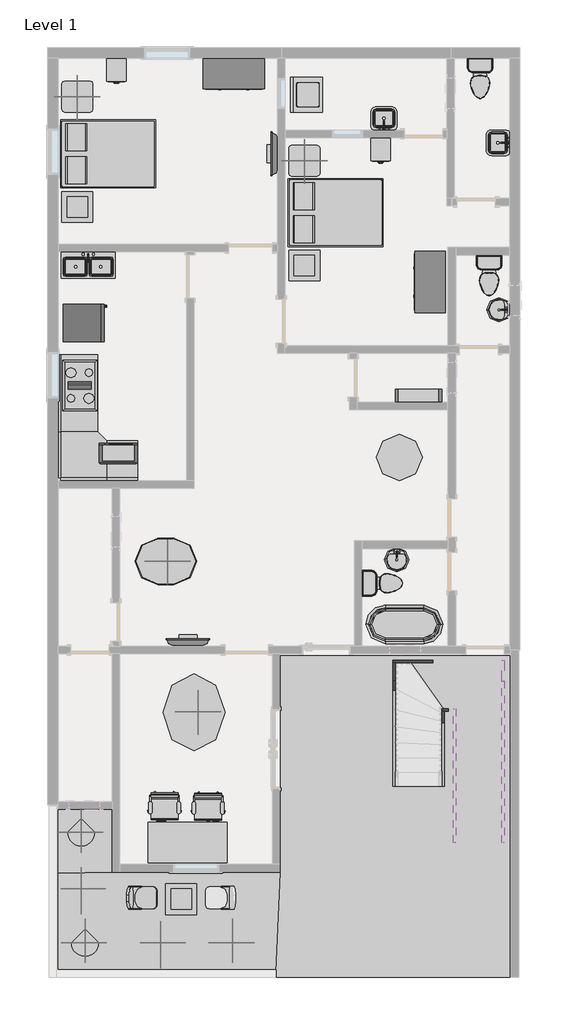
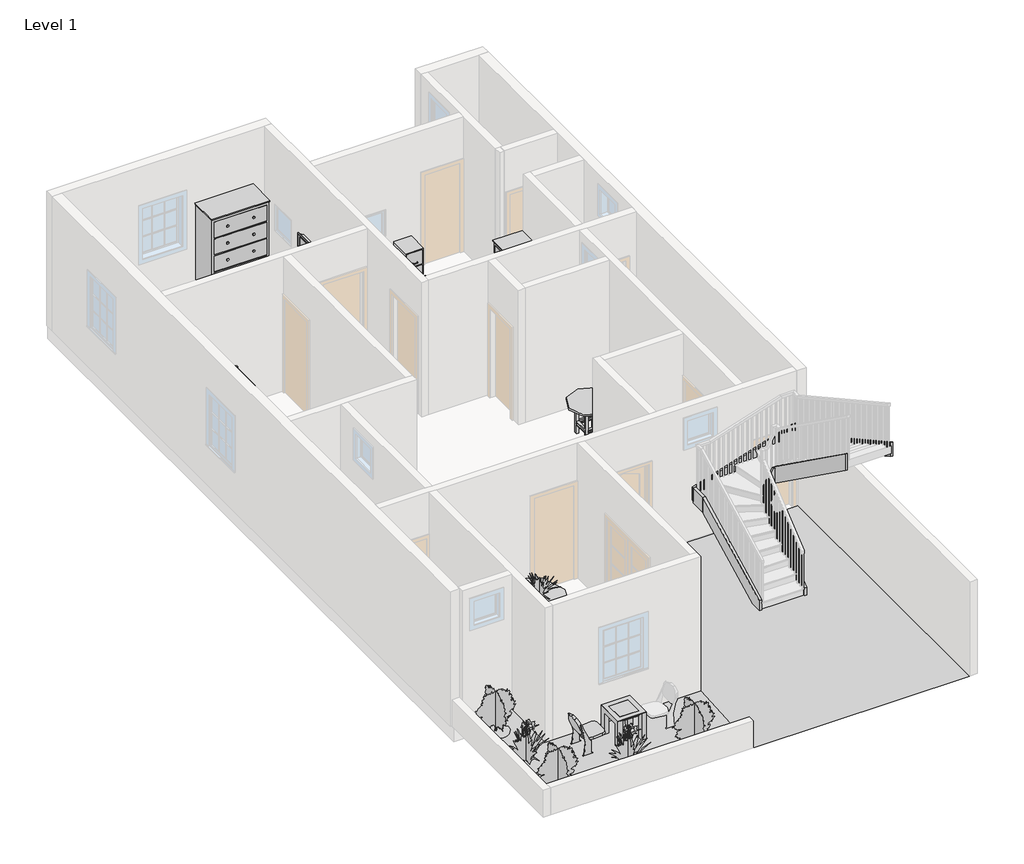
# One storey, part 3 of 3: 22 furniture elements, 13 flow terminals, 9 geographic elements, 8 members, 7 proxies.
"""IFC4 building model written with IfcOpenShell, lengths in millimetres."""

from ifc_helpers import new_model, si_unit, frame, origin, place, context, project, spatial, polyline, outline, extrude, triangles, transform, mapped, element, save
from components import proxy_bb1e6e30, proxy_8a8d5ab2, proxy_a13a33b2, proxy_718fa39f, flow_terminal_accce45a, flow_terminal_a53be723, flow_terminal_d49f872f, flow_terminal_62a433f7, toilet_domestic_3d_toilet_domestic_3d_f7549cf7, toilet_domestic_3d_toilet_domestic_3d_183bbd19, flow_terminal_b374fae2, furniture_c8abb964, furniture_bb55ed6b, chair_task_arms_chair_task_arms_fa5a08ef, furniture_072f6425, furniture_9fa109b2, furniture_3d1d9cbc, furniture_417d203a, furniture_56245f3a, furniture_b5c51a22, furniture_be1c6672, furniture_905aceb5, furniture_743965d2, furniture_31d08a24, furniture_be658349, rpc_plant_tropical_55f6ff97, rpc_plant_tropical_agave_1_5_93a2a214, rpc_plant_tropical_jungle_flame_3_9c4808c2

model = new_model("IFC4")

# Units and contexts
model_context = context("Model", 3, world=origin())
ifc_project = project(units=[si_unit("LENGTHUNIT", "METRE", prefix="MILLI")], contexts=[model_context])

# Site, building, storey
site = spatial("IfcSite", under=ifc_project)
building = spatial("IfcBuilding", under=site)
storey = spatial("IfcBuildingStorey", under=building, Name="Level 1", Elevation=0.0)

# Proxies
placement = place(None, origin())
element("IfcBuildingElementProxy", 1, Name="Building Element Proxy", at=placement, inside=storey, context=model_context, shape_type="Tessellation", body=[
    triangles([(-14477.8023376, -2094.7895782, 0.0), (-13411.0023376, -2094.7895782, 0.0), (-13411.0023376, -3339.3894814, 0.0), (-14477.8023376, -3385.7244438, 0.0)], [[1, 4, 3], [3, 2, 1]], closed=False),
])
element("IfcBuildingElementProxy", 2, Name="Building Element Proxy", at=placement, inside=storey, context=model_context, shape_type="Tessellation", body=[
    triangles([(-14477.8023376, -5320.589772, 0.0), (-10171.4268219, -5320.589772, 0.0), (-10083.6019501, -3339.3894814, 0.0), (-14477.8023376, -3358.5089539, 0.0), (-13411.0023376, -3339.3894814, 0.0)], [[4, 1, 5], [5, 2, 3], [2, 5, 1]], closed=False),
])
element("IfcBuildingElementProxy", 3, Name="Building Element Proxy", at=placement, inside=storey, context=model_context, shape_type="Tessellation", body=[
    triangles([(-10083.6019501, 978.6103975, 0.0), (-5537.0021439, 978.6103975, 0.0), (-5537.0021439, -5422.1893845, 0.0), (-10159.8019501, -5422.1893845, 0.0), (-9613.7021439, 1061.1603733, 0.0), (-5613.2021439, 1080.2103733, 0.0)], [[4, 5, 1], [5, 4, 3], [5, 2, 6], [2, 5, 3]], closed=False),
])
proxy_shape = proxy_bb1e6e30(model_context)
element("IfcBuildingElementProxy", 4, Name="Cook Top-4 Unit : 36\" x 20\"", ObjectType="Cook Top-4 Unit : 36\" x 20\"", at=placement, inside=storey, context=model_context, shape_type="MappedRepresentation", body=[
    mapped(proxy_shape, transform((-14046.0021832, 6287.2104001, 0.0), x_axis=(0.0, 1.0000000000000002, 0.0), y_axis=(-1.0000000000000002, 0.0, 0.0), z_axis=(0.0, 0.0, 1.0))),
])
proxy_2_shape = proxy_8a8d5ab2(model_context)
element("IfcBuildingElementProxy", 5, Name="Microwave : 30\" x 16\" x 18\"", ObjectType="Microwave : 30\" x 16\" x 18\"", at=placement, inside=storey, context=model_context, shape_type="MappedRepresentation", body=[
    mapped(proxy_2_shape, transform((-12783.7093059, 4587.9298943, 0.0), x_axis=(-1.0000000000000004, 0.0, 0.0), y_axis=(0.0, -1.0000000000000004, 0.0), z_axis=(0.0, 0.0, 1.0))),
])
proxy_3_shape = proxy_a13a33b2(model_context)
element("IfcBuildingElementProxy", 6, Name="Refrigerator : 30\" x 32\" RH", ObjectType="Refrigerator : 30\" x 32\" RH", at=placement, inside=storey, context=model_context, shape_type="MappedRepresentation", body=[
    mapped(proxy_3_shape, transform((-13987.2646832, 7524.2614286, 0.0), x_axis=(0.0, 1.0000000000000004, 0.0), y_axis=(-1.0000000000000004, 0.0, 0.0), z_axis=(0.0, 0.0, 1.0))),
])
proxy_4_shape = proxy_718fa39f(model_context)
element("IfcBuildingElementProxy", 7, Name="Washer : 27\" x 25\" x 35\"", ObjectType="Washer : 27\" x 25\" x 35\"", at=placement, inside=storey, context=model_context, shape_type="MappedRepresentation", body=[
    mapped(proxy_4_shape, transform((-9283.7526184, 11619.8929316, 0.0), x_axis=(0.0, 1.0000000000000004, 0.0), y_axis=(-1.0000000000000004, 0.0, 0.0), z_axis=(0.0, 0.0, 1.0))),
])

# Flow terminals
flow_terminal_shape = flow_terminal_accce45a(model_context)
element("IfcFlowTerminal", 8, ObjectType="Floor Drain - Round : 5\" Strainer - 2\" Drain", at=placement, inside=storey, context=model_context, shape_type="MappedRepresentation", body=[
    mapped(flow_terminal_shape, transform((-9042.2021832, 12611.8104001, 0.0), x_axis=(1.0, 0.0, 0.0), y_axis=(0.0, 1.0, 0.0), z_axis=(0.0, 0.0, 1.0))),
])
element("IfcFlowTerminal", 9, ObjectType="Floor Drain - Round : 5\" Strainer - 2\" Drain", at=placement, inside=storey, context=model_context, shape_type="MappedRepresentation", body=[
    mapped(flow_terminal_shape, transform((-5689.4021832, 11951.4104001, 0.0), x_axis=(1.0, 0.0, 0.0), y_axis=(0.0, 1.0, 0.0), z_axis=(0.0, 0.0, 1.0))),
])
element("IfcFlowTerminal", 10, ObjectType="Floor Drain - Round : 5\" Strainer - 2\" Drain", at=placement, inside=storey, context=model_context, shape_type="MappedRepresentation", body=[
    mapped(flow_terminal_shape, transform((-6444.5985247, 8407.5245964, 0.0), x_axis=(1.0, 0.0, 0.0), y_axis=(0.0, 1.0, 0.0), z_axis=(0.0, 0.0, 1.0))),
])
element("IfcFlowTerminal", 11, ObjectType="Floor Drain - Round : 5\" Strainer - 2\" Drain", at=placement, inside=storey, context=model_context, shape_type="MappedRepresentation", body=[
    mapped(flow_terminal_shape, transform((-8077.0021832, 2070.8104001, 0.0), x_axis=(1.0, 0.0, 0.0), y_axis=(0.0, 1.0, 0.0), z_axis=(0.0, 0.0, 1.0))),
])
flow_terminal_2_shape = flow_terminal_a53be723(model_context)
element("IfcFlowTerminal", 12, ObjectType="Sink Kitchen-Double : 42\" x 21\"", at=placement, inside=storey, context=model_context, shape_type="MappedRepresentation", body=[
    mapped(flow_terminal_2_shape, transform((-13896.5914237, 8672.464999, 0.0), x_axis=(1.0, 0.0, 0.0), y_axis=(0.0, 1.0, 0.0), z_axis=(0.0, 0.0, 1.0))),
])
flow_terminal_3_shape = flow_terminal_d49f872f(model_context)
element("IfcFlowTerminal", 13, ObjectType="Sink Vanity-Round : 19\" x 19\"", at=placement, inside=storey, context=model_context, shape_type="MappedRepresentation", body=[
    mapped(flow_terminal_3_shape, transform((-5832.6532538, 7882.4621407, 0.0), x_axis=(0.0, -1.0000000000000002, 0.0), y_axis=(1.0000000000000002, 0.0, 0.0), z_axis=(0.0, 0.0, 1.0))),
])
element("IfcFlowTerminal", 14, ObjectType="Sink Vanity-Round : 19\" x 19\"", at=placement, inside=storey, context=model_context, shape_type="MappedRepresentation", body=[
    mapped(flow_terminal_3_shape, transform((-7868.8539237, 2754.6268451, 0.0), x_axis=(1.0, 0.0, 0.0), y_axis=(0.0, 1.0, 0.0), z_axis=(0.0, 0.0, 1.0))),
])
flow_terminal_4_shape = flow_terminal_62a433f7(model_context)
element("IfcFlowTerminal", 15, ObjectType="Sink Vanity-Square : 20\" x 18\"", at=placement, inside=storey, context=model_context, shape_type="MappedRepresentation", body=[
    mapped(flow_terminal_4_shape, transform((-8010.5129426, 11521.9558012, 0.0), x_axis=(-1.0, 0.0, 0.0), y_axis=(0.0, -1.0, 0.0), z_axis=(0.0, 0.0, 1.0))),
])
element("IfcFlowTerminal", 16, ObjectType="Sink Vanity-Square : 20\" x 18\"", at=placement, inside=storey, context=model_context, shape_type="MappedRepresentation", body=[
    mapped(flow_terminal_4_shape, transform((-5717.1475843, 11103.4996407, 0.0), x_axis=(0.0, -1.0, 0.0), y_axis=(1.0, 0.0, 0.0), z_axis=(0.0, 0.0, 1.0))),
])
toilet_domestic_3d_toilet_domestic_3d_shape = toilet_domestic_3d_toilet_domestic_3d_f7549cf7(model_context)
toilet_domestic_3d_toilet_domestic_3d_2_shape = toilet_domestic_3d_toilet_domestic_3d_183bbd19(model_context)
element("IfcFlowTerminal", 17, ObjectType="Toilet-Domestic-3D : Toilet-Domestic-3D", at=placement, inside=storey, context=model_context, shape_type="MappedRepresentation", body=[
    mapped(toilet_domestic_3d_toilet_domestic_3d_shape, transform((-6121.2021832, 12269.5143727, 0.0), x_axis=(1.0, 0.0, 0.0), y_axis=(0.0, 1.0, 0.0), z_axis=(0.0, 0.0, 1.0))),
    mapped(toilet_domestic_3d_toilet_domestic_3d_2_shape, transform((-6121.2021832, 12269.5143727, 0.0), x_axis=(1.0, 0.0, 0.0), y_axis=(0.0, 1.0, 0.0), z_axis=(0.0, 0.0, 1.0))),
])
element("IfcFlowTerminal", 18, ObjectType="Toilet-Domestic-3D : Toilet-Domestic-3D", at=placement, inside=storey, context=model_context, shape_type="MappedRepresentation", body=[
    mapped(toilet_domestic_3d_toilet_domestic_3d_shape, transform((-5943.4021832, 8370.0104001, 0.0), x_axis=(1.0, 0.0, 0.0), y_axis=(0.0, 1.0, 0.0), z_axis=(0.0, 0.0, 1.0))),
    mapped(toilet_domestic_3d_toilet_domestic_3d_2_shape, transform((-5943.4021832, 8370.0104001, 0.0), x_axis=(1.0, 0.0, 0.0), y_axis=(0.0, 1.0, 0.0), z_axis=(0.0, 0.0, 1.0))),
])
element("IfcFlowTerminal", 19, ObjectType="Toilet-Domestic-3D : Toilet-Domestic-3D", at=placement, inside=storey, context=model_context, shape_type="MappedRepresentation", body=[
    mapped(toilet_domestic_3d_toilet_domestic_3d_shape, transform((-7963.3061558, 2375.6104001, 0.0), x_axis=(0.0, 1.0000000000000002, 0.0), y_axis=(-1.0000000000000002, 0.0, 0.0), z_axis=(0.0, 0.0, 1.0))),
    mapped(toilet_domestic_3d_toilet_domestic_3d_2_shape, transform((-7963.3061558, 2375.6104001, 0.0), x_axis=(0.0, 1.0000000000000002, 0.0), y_axis=(-1.0000000000000002, 0.0, 0.0), z_axis=(0.0, 0.0, 1.0))),
])
flow_terminal_5_shape = flow_terminal_b374fae2(model_context)
element("IfcFlowTerminal", 20, ObjectType="Tub-Free Standing-3D : 30\" x 60\"", at=placement, inside=storey, context=model_context, shape_type="MappedRepresentation", body=[
    mapped(flow_terminal_5_shape, transform((-7619.8021832, 1562.8104001, 0.0), x_axis=(0.0, 1.0000000000000002, 0.0), y_axis=(-1.0000000000000002, 0.0, 0.0), z_axis=(0.0, 0.0, 1.0))),
])

# Furniture
furniture_shape = furniture_c8abb964(model_context)
element("IfcFurniture", 21, ObjectType="Bed-Box : Double 53\" x 74\"", at=placement, inside=storey, context=model_context, shape_type="MappedRepresentation", body=[
    mapped(furniture_shape, transform((-13721.6316914, 10532.7579411, 0.0), x_axis=(0.0, 1.0, 0.0), y_axis=(-1.0, 0.0, 0.0), z_axis=(0.0, 0.0, 1.0))),
])
element("IfcFurniture", 22, ObjectType="Bed-Box : Double 53\" x 74\"", at=placement, inside=storey, context=model_context, shape_type="MappedRepresentation", body=[
    mapped(furniture_shape, transform((-9216.2546422, 9366.4399083, 0.0), x_axis=(0.0, 1.0000000000000002, 0.0), y_axis=(-1.0000000000000002, 0.0, 0.0), z_axis=(0.0, 0.0, 1.0))),
])
furniture_2_shape = furniture_bb55ed6b(model_context)
element("IfcFurniture", 23, ObjectType="Cabinet-File 2 Drawer : 15\" x 18\"", at=placement, inside=storey, context=model_context, shape_type="MappedRepresentation", body=[
    mapped(furniture_2_shape, transform((-13194.2057361, 12677.7447002, 0.0), x_axis=(1.0, 0.0, 0.0), y_axis=(0.0, 1.0, 0.0), z_axis=(0.0, 0.0, 1.0))),
])
element("IfcFurniture", 24, ObjectType="Cabinet-File 2 Drawer : 15\" x 18\"", at=placement, inside=storey, context=model_context, shape_type="MappedRepresentation", body=[
    mapped(furniture_2_shape, transform((-7961.8057361, 11102.9447002, 0.0), x_axis=(1.0, 0.0, 0.0), y_axis=(0.0, 1.0, 0.0), z_axis=(0.0, 0.0, 1.0))),
])
chair_task_arms_chair_task_arms_shape = chair_task_arms_chair_task_arms_fa5a08ef(model_context)
element("IfcFurniture", 25, ObjectType="Chair-Task Arms : Chair-Task Arms", at=placement, inside=storey, context=model_context, shape_type="MappedRepresentation", body=[
    mapped(chair_task_arms_chair_task_arms_shape, transform((-12228.6113635, -2018.6936983, 0.0), x_axis=(-1.0000000000000004, 0.0, 0.0), y_axis=(0.0, -1.0000000000000004, 0.0), z_axis=(0.0, 0.0, 1.0))),
])
element("IfcFurniture", 26, ObjectType="Chair-Task Arms : Chair-Task Arms", at=placement, inside=storey, context=model_context, shape_type="MappedRepresentation", body=[
    mapped(chair_task_arms_chair_task_arms_shape, transform((-11365.0113635, -2025.0436983, 0.0), x_axis=(-1.0000000000000004, 0.0, 0.0), y_axis=(0.0, -1.0000000000000004, 0.0), z_axis=(0.0, 0.0, 1.0))),
])
furniture_3_shape = furniture_072f6425(model_context)
element("IfcFurniture", 27, ObjectType="Desk : 60\" x 30\" Student", at=placement, inside=storey, context=model_context, shape_type="MappedRepresentation", body=[
    mapped(furniture_3_shape, transform((-12674.4021832, -3136.1895999, 0.0), x_axis=(1.0000000000000009, 0.0, 0.0), y_axis=(0.0, 1.0000000000000009, 0.0), z_axis=(0.0, 0.0, 1.0))),
])
furniture_4_shape = furniture_9fa109b2(model_context)
element("IfcFurniture", 28, ObjectType="Dresser : 48\" x 72\" x 24\"", at=placement, inside=storey, context=model_context, shape_type="MappedRepresentation", body=[
    mapped(furniture_4_shape, transform((-10728.8089233, 12822.5733542, 0.0), x_axis=(1.0, 0.0, 0.0), y_axis=(0.0, 1.0, 0.0), z_axis=(0.0, 0.0, 1.0))),
])
element("IfcFurniture", 29, ObjectType="Dresser : 48\" x 72\" x 24\"", at=placement, inside=storey, context=model_context, shape_type="MappedRepresentation", body=[
    mapped(furniture_4_shape, transform((-6748.6392291, 8062.7171403, 0.0), x_axis=(0.0, -1.0000000000000007, 0.0), y_axis=(1.0000000000000007, 0.0, 0.0), z_axis=(0.0, 0.0, 1.0))),
])
furniture_5_shape = furniture_3d1d9cbc(model_context)
element("IfcFurniture", 30, ObjectType="Seating-Auditorium : 18\" x 24\" x 30\"", at=placement, inside=storey, context=model_context, shape_type="MappedRepresentation", body=[
    mapped(furniture_5_shape, transform((-13016.677593, -3686.661731, 0.0), x_axis=(0.0, -1.0000000000000004, 0.0), y_axis=(1.0000000000000004, 0.0, 0.0), z_axis=(0.0, 0.0, 1.0))),
])
furniture_6_shape = furniture_417d203a(model_context)
element("IfcFurniture", 31, ObjectType="Shelving : 36\" x 10\" x 72\"", at=placement, inside=storey, context=model_context, shape_type="MappedRepresentation", body=[
    mapped(furniture_6_shape, transform((-7340.4021832, 5779.2104001, 0.0), x_axis=(-1.0, 0.0, 0.0), y_axis=(0.0, -1.0, 0.0), z_axis=(0.0, 0.0, 1.0))),
])
furniture_7_shape = furniture_56245f3a(model_context)
element("IfcFurniture", 32, ObjectType="TV - Flat Screen : 32\"", at=placement, inside=storey, context=model_context, shape_type="MappedRepresentation", body=[
    mapped(furniture_7_shape, transform((-10192.9408068, 10867.965886, 990.6), x_axis=(0.0, -1.0000000000000004, 0.0), y_axis=(1.0000000000000004, 0.0, 0.0), z_axis=(0.0, 0.0, 1.0))),
])
element("IfcFurniture", 33, ObjectType="TV - Flat Screen : 32\"", at=placement, inside=storey, context=model_context, shape_type="MappedRepresentation", body=[
    mapped(furniture_7_shape, transform((-11909.9966973, 1208.5990237, 990.6), x_axis=(-1.0, 0.0, 0.0), y_axis=(0.0, -1.0, 0.0), z_axis=(0.0, 0.0, 1.0))),
])
furniture_8_shape = furniture_b5c51a22(model_context)
element("IfcFurniture", 34, ObjectType="Table-Coffee : 24\" x 24\" x 24\"", at=placement, inside=storey, context=model_context, shape_type="MappedRepresentation", body=[
    mapped(furniture_8_shape, transform((-14115.0679499, 9722.5993223, 0.0), x_axis=(1.0, 0.0, 0.0), y_axis=(0.0, 1.0, 0.0), z_axis=(0.0, 0.0, 1.0))),
])
element("IfcFurniture", 35, ObjectType="Table-Coffee : 24\" x 24\" x 24\"", at=placement, inside=storey, context=model_context, shape_type="MappedRepresentation", body=[
    mapped(furniture_8_shape, transform((-9619.2679499, 8566.8993223, 0.0), x_axis=(1.0, 0.0, 0.0), y_axis=(0.0, 1.0, 0.0), z_axis=(0.0, 0.0, 1.0))),
])
element("IfcFurniture", 36, ObjectType="Table-Coffee : 24\" x 24\" x 24\"", at=placement, inside=storey, context=model_context, shape_type="MappedRepresentation", body=[
    mapped(furniture_8_shape, transform((-12057.6679499, -3968.0006777, 0.0), x_axis=(1.0, 0.0, 0.0), y_axis=(0.0, 1.0, 0.0), z_axis=(0.0, 0.0, 1.0))),
])
furniture_9_shape = furniture_be1c6672(model_context)
element("IfcFurniture", 37, ObjectType="Table-Dining Oval : 36\" x 48\"", at=placement, inside=storey, context=model_context, shape_type="MappedRepresentation", body=[
    mapped(furniture_9_shape, transform((-11942.3825111, 3165.5087608, 0.0), x_axis=(1.0, 0.0, 0.0), y_axis=(0.0, 1.0, 0.0), z_axis=(0.0, 0.0, 1.0))),
])
furniture_10_shape = furniture_905aceb5(model_context)
element("IfcFurniture", 38, ObjectType="Table-Dining Round w Chairs : 36\" Diameter", at=placement, inside=storey, context=model_context, shape_type="MappedRepresentation", body=[
    mapped(furniture_10_shape, transform((-7825.0841504, 5049.6890886, 0.0), x_axis=(1.0, 0.0, 0.0), y_axis=(0.0, 1.0, 0.0), z_axis=(0.0, 0.0, 1.0))),
])
furniture_11_shape = furniture_743965d2(model_context)
element("IfcFurniture", 39, ObjectType="Table-Ellipse : 60\" x 48\"", at=placement, inside=storey, context=model_context, shape_type="MappedRepresentation", body=[
    mapped(furniture_11_shape, transform((-11785.4021832, -177.0895999, 0.0), x_axis=(0.0, 1.0, 0.0), y_axis=(-1.0, 0.0, 0.0), z_axis=(0.0, 0.0, 1.0))),
])
furniture_12_shape = furniture_31d08a24(model_context)
element("IfcFurniture", 40, ObjectType="Table-End : 24\" x 24\"", at=placement, inside=storey, context=model_context, shape_type="MappedRepresentation", body=[
    mapped(furniture_12_shape, transform((-14405.3358135, 11849.8104001, 0.0), x_axis=(1.0, 0.0, 0.0), y_axis=(0.0, 1.0, 0.0), z_axis=(0.0, 0.0, 1.0))),
])
element("IfcFurniture", 41, ObjectType="Table-End : 24\" x 24\"", at=placement, inside=storey, context=model_context, shape_type="MappedRepresentation", body=[
    mapped(furniture_12_shape, transform((-9909.5358135, 10579.8104001, 0.0), x_axis=(1.0, 0.0, 0.0), y_axis=(0.0, 1.0, 0.0), z_axis=(0.0, 0.0, 1.0))),
])
furniture_13_shape = furniture_be658349(model_context)
element("IfcFurniture", 42, ObjectType="Work Station Cubicle : 96\" x 96\"", at=placement, inside=storey, context=model_context, shape_type="MappedRepresentation", body=[
    mapped(furniture_13_shape, transform((-14972.8251908, 4539.3421523, 0.0), x_axis=(0.0, 1.0000000000000002, 0.0), y_axis=(-1.0000000000000002, 0.0, 0.0), z_axis=(0.0, 0.0, 1.0))),
])

# Geographic elements
rpc_plant_tropical_shape = rpc_plant_tropical_55f6ff97(model_context)
element("IfcGeographicElement", 43, ObjectType="RPC Plant - Tropical", at=placement, inside=storey, context=model_context, shape_type="MappedRepresentation", body=[
    mapped(rpc_plant_tropical_shape, transform((-14020.6021832, -3669.5895999, 0.0), x_axis=(1.0, 0.0, 0.0), y_axis=(0.0, 1.0, 0.0), z_axis=(0.0, 0.0, 1.0))),
])
element("IfcGeographicElement", 44, ObjectType="RPC Plant - Tropical", at=placement, inside=storey, context=model_context, shape_type="MappedRepresentation", body=[
    mapped(rpc_plant_tropical_shape, transform((-12445.8021832, -4736.3895999, 0.0), x_axis=(1.0, 0.0, 0.0), y_axis=(0.0, 1.0, 0.0), z_axis=(0.0, 0.0, 1.0))),
])
rpc_plant_tropical_agave_1_5_shape = rpc_plant_tropical_agave_1_5_93a2a214(model_context)
element("IfcGeographicElement", 45, ObjectType="RPC Plant - Tropical : Agave - 1.5'", at=placement, inside=storey, context=model_context, shape_type="MappedRepresentation", body=[
    mapped(rpc_plant_tropical_agave_1_5_shape, transform((-14096.8021832, 12002.2104001, 609.6), x_axis=(1.0, 0.0, 0.0), y_axis=(0.0, 1.0, 0.0), z_axis=(0.0, 0.0, 1.0))),
])
element("IfcGeographicElement", 46, ObjectType="RPC Plant - Tropical : Agave - 1.5'", at=placement, inside=storey, context=model_context, shape_type="MappedRepresentation", body=[
    mapped(rpc_plant_tropical_agave_1_5_shape, transform((-9601.0021832, 10732.2104001, 609.6), x_axis=(1.0, 0.0, 0.0), y_axis=(0.0, 1.0, 0.0), z_axis=(0.0, 0.0, 1.0))),
])
element("IfcGeographicElement", 47, ObjectType="RPC Plant - Tropical : Agave - 1.5'", at=placement, inside=storey, context=model_context, shape_type="MappedRepresentation", body=[
    mapped(rpc_plant_tropical_agave_1_5_shape, transform((-12306.1021832, 2807.4104001, 609.6), x_axis=(1.0, 0.0, 0.0), y_axis=(0.0, 1.0, 0.0), z_axis=(0.0, 0.0, 1.0))),
])
element("IfcGeographicElement", 48, ObjectType="RPC Plant - Tropical : Agave - 1.5'", at=placement, inside=storey, context=model_context, shape_type="MappedRepresentation", body=[
    mapped(rpc_plant_tropical_agave_1_5_shape, transform((-11709.2021832, -164.3895999, 762.0), x_axis=(1.0, 0.0, 0.0), y_axis=(0.0, 1.0, 0.0), z_axis=(0.0, 0.0, 1.0))),
])
rpc_plant_tropical_jungle_flame_3_shape = rpc_plant_tropical_jungle_flame_3_9c4808c2(model_context)
element("IfcGeographicElement", 49, ObjectType="RPC Plant - Tropical : Jungle Flame - 3'", at=placement, inside=storey, context=model_context, shape_type="MappedRepresentation", body=[
    mapped(rpc_plant_tropical_jungle_flame_3_shape, transform((-14020.6021832, -2551.9895999, 0.0), x_axis=(1.0, 0.0, 0.0), y_axis=(0.0, 1.0, 0.0), z_axis=(0.0, 0.0, 1.0))),
])
element("IfcGeographicElement", 50, ObjectType="RPC Plant - Tropical : Jungle Flame - 3'", at=placement, inside=storey, context=model_context, shape_type="MappedRepresentation", body=[
    mapped(rpc_plant_tropical_jungle_flame_3_shape, transform((-13944.4021832, -4736.3895999, 0.0), x_axis=(1.0, 0.0, 0.0), y_axis=(0.0, 1.0, 0.0), z_axis=(0.0, 0.0, 1.0))),
])
element("IfcGeographicElement", 51, ObjectType="RPC Plant - Tropical : Jungle Flame - 3'", at=placement, inside=storey, context=model_context, shape_type="MappedRepresentation", body=[
    mapped(rpc_plant_tropical_jungle_flame_3_shape, transform((-11023.4021832, -4736.3895999, 0.0), x_axis=(1.0, 0.0, 0.0), y_axis=(0.0, 1.0, 0.0), z_axis=(0.0, 0.0, 1.0))),
])

# Members
element("IfcMember", 52, ObjectType="Stringer - 2\" Width", at=placement, inside=storey, context=model_context, shape_type="SweptSolid", body=[
    extrude(outline(polyline([(-1637.5895999, 0.0), (-1637.5895999, 229.639954), (449.8275918, 1305.3956453), (449.8275918, 962.500629), (-1417.8272823, 0.0), (-1637.5895999, 0.0)])), frame((-7848.4021832, 0.0, 0.0), z_axis=(1.0, 0.0, 0.0), x_axis=(0.0, 1.0, 0.0)), (0.0, 0.0, 1.0), 50.8),
])
element("IfcMember", 53, ObjectType="Stringer - 2\" Width", at=placement, inside=storey, context=model_context, shape_type="SweptSolid", body=[
    extrude(outline(polyline([(-7797.6021832, 449.8275918), (-7848.4021832, 449.8275918), (-7848.4021832, 804.542092), (-7797.6021832, 804.542092), (-7797.6021832, 449.8275918)])), frame((0.0, 0.0, 962.500629), z_axis=(0.0, 0.0, 1.0), x_axis=(1.0, 0.0, 0.0)), (0.0, 0.0, 1.0), 342.8950162),
])
element("IfcMember", 54, ObjectType="Stringer - 2\" Width", at=placement, inside=storey, context=model_context, shape_type="SweptSolid", body=[
    extrude(outline(polyline([(1289.0952212, -7848.4021832), (1000.5956453, -7848.4021832), (1000.5956453, -7678.8797002), (1638.9682298, -5689.4021832), (1969.9972697, -5689.4021832), (1969.9972697, -5726.3823005), (1289.0952212, -7848.4021832)])), frame((0.0, 804.542092, 0.0), z_axis=(0.0, 1.0, 0.0), x_axis=(0.0, 0.0, 1.0)), (0.0, 0.0, 1.0), 50.8),
])
element("IfcMember", 55, ObjectType="Stringer - 2\" Width", at=placement, inside=storey, context=model_context, shape_type="SweptSolid", body=[
    extrude(outline(polyline([(-5689.4021832, 855.342092), (-5638.6021832, 855.342092), (-5638.6021832, 438.8433457), (-5689.4021832, 438.8433457), (-5689.4021832, 855.342092)])), frame((0.0, 0.0, 1649.8904473), z_axis=(0.0, 0.0, 1.0), x_axis=(1.0, 0.0, 0.0)), (0.0, 0.0, 1.0), 320.1068224),
])
element("IfcMember", 56, ObjectType="Stringer - 2\" Width", at=placement, inside=storey, context=model_context, shape_type="SweptSolid", body=[
    extrude(outline(polyline([(438.8433457, 1969.9972697), (438.8433457, 1649.8904473), (-2755.1895999, 3413.2400755), (-2755.1895999, 3733.3468979), (438.8433457, 1969.9972697)])), frame((-5689.4021832, 0.0, 0.0), z_axis=(1.0, 0.0, 0.0), x_axis=(0.0, 1.0, 0.0)), (0.0, 0.0, 1.0), 50.8),
])
element("IfcMember", 57, ObjectType="Stringer - 2\" Width", at=placement, inside=storey, context=model_context, shape_type="SweptSolid", body=[
    extrude(outline(polyline([(-1637.5895999, 0.0), (-1637.5895999, 176.1764461), (-160.657908, 1380.418648), (-160.657908, 987.1410923), (-1371.3279553, 0.0), (-1637.5895999, 0.0)])), frame((-6883.2021832, 0.0, 0.0), z_axis=(1.0, 0.0, 0.0), x_axis=(0.0, 1.0, 0.0)), (0.0, 0.0, 1.0), 50.8),
])
element("IfcMember", 58, ObjectType="Stringer - 2\" Width", at=placement, inside=storey, context=model_context, shape_type="SweptSolid", body=[
    extrude(outline(polyline([(1573.2682978, -6883.2021832), (1028.5617647, -6883.2021832), (1028.5617647, -6848.9599659), (1360.465107, -6654.6021832), (1914.9943794, -6654.6021832), (1914.9943794, -6683.0923469), (1573.2682978, -6883.2021832)])), frame((0.0, -160.657908, 0.0), z_axis=(0.0, 1.0, 0.0), x_axis=(0.0, 0.0, 1.0)), (0.0, 0.0, 1.0), 50.8),
])
element("IfcMember", 59, ObjectType="Stringer - 2\" Width", at=placement, inside=storey, context=model_context, shape_type="SweptSolid", body=[
    extrude(outline(polyline([(-109.857908, 1914.9943794), (-109.857908, 1540.0492775), (-2755.1895999, 3435.1700453), (-2755.1895999, 3810.1151472), (-109.857908, 1914.9943794)])), frame((-6654.6021832, 0.0, 0.0), z_axis=(1.0, 0.0, 0.0), x_axis=(0.0, 1.0, 0.0)), (0.0, 0.0, 1.0), 50.8),
])

save(model, "model.ifc")

# Revit data of these elements
# Type "Cook Top-4 Unit : 36\" x 20\""
#   Assembly Code = "E1090400"
#   Depth = 2' - 0"
#   Width = 3' - 0"
#   Burner Material = Steel, Chrome Plated
#   Cooktop Material = Steel, Polished
#   Default Elevation = 0
# Type "Microwave : 30\" x 16\" x 18\""
#   Assembly Code = "E1090400"
#   Depth = 1' - 4"
#   Height = 1' - 6"
#   Width = 2' - 6"
#   Microwave Material = Laminate, Ivory, Matte
#   Default Elevation = 0
# Type "Refrigerator : 30\" x 32\" RH"
#   Label = "REF."
#   Assembly Code = "E1090400"
#   Depth = 2' - 7 3/4"
#   Handle = 2' - 3"
#   Height = 5' - 10"
#   Rear Clearance = 0' - 2"
#   Top Door Height = 1' - 8"
#   Width = 2' - 5 3/8"
#   Material = Steel, Paint Finish, Ivory, Glossy
#   Default Elevation = 0
# Type "Washer : 27\" x 25\" x 35\""
#   Label = "W"
#   Assembly Code = "E1090400"
#   Depth = 2' - 1"
#   Height = 2' - 11"
#   Width = 2' - 3"
#   Washer Material = Steel, Paint Finish, Ivory, Matte
#   Default Elevation = 0
# Type "Floor Drain - Round : 5\" Strainer - 2\" Drain"
#   WFU = 2
#   Strainer Height = 0' - 3 1/4"
#   Strainer Radius = 0' - 2 1/2"
#   Strainer Diameter = 0' - 5"
#   Radius 6 = 0' - 0 5/8"
#   Radius 5 = 0' - 1 1/4"
#   Radius 4 = 0' - 1 7/8"
#   Radius 2 = 0' - 3.04167"
#   Radius 1 = 0' - 2.02083"
#   Radius 3 = 0' - 2 1/32"
#   Pipe Radius = 1"
#   Pipe Diameter = 2"
#   Height 2 = 0' - 0.725"
#   Height 1 = 0' - 1 13/16"
#   Body Radius = 0' - 4 1/16"
#   Body Height = 0' - 3 5/8"
#   Body Diameter = 0' - 8 1/8"
#   Drain Material = none
#   HWFU = 0
#   Default Elevation = 0
#   CWFU = 0
# Type "Sink Kitchen-Double : 42\" x 21\""
#   Assembly Code = "D2010410"
#   Counter Height = 3' - 0"
#   Depth = 1' - 9"
#   Width = 3' - 6"
#   Faucet Material = Steel, Polished
#   Sink Material = Steel, Polished
#   Default Elevation = 0
# Type "Sink Vanity-Round : 19\" x 19\""
#   Assembly Code = "D2010400"
#   Top Of Counter = 2' - 7"
#   Basin Material = Porcelain, Linen
#   Faucet Material = Steel, Polished
#   Default Elevation = 0
# Type "Sink Vanity-Square : 20\" x 18\""
#   Assembly Code = "D2010400"
#   Counter Height = 2' - 7"
#   Depth = 1' - 6"
#   Width = 1' - 8"
#   Basin Material = Porcelain, Linen
#   Faucet Material = Steel, Polished
#   Default Elevation = 0
# Type "Toilet-Domestic-3D : Toilet-Domestic-3D"
#   Assembly Code = "D2010110"
#   Toilet - Bowl/Basin Material = Porcelain, Linen
#   Toilet - Seat Material = Laminate, Linen, Matte
#   Default Elevation = 0
# Type "Tub-Free Standing-3D : 30\" x 60\""
#   Assembly Code = "D2010110"
#   Height = 1' - 6"
#   Length = 5' - 0"
#   Width = 2' - 6"
#   Tub Material = Porcelain, Ivory
#   Default Elevation = 0
# Type "Bed-Box : Double 53\" x 74\""
#   Assembly Code = "E2020200"
#   Length = 6' - 2"
#   Width = 4' - 5"
#   Frame Material = Birch
#   Mattress Material = Linen, White
#   Default Elevation = 0
# Type "Cabinet-File 2 Drawer : 15\" x 18\""
#   Assembly Code = "E2020200"
#   Depth = 1' - 6"
#   Height = 2' - 5"
#   Width = 1' - 3"
#   Cabinet Material = Steel, Paint Finish, Ivory, Glossy
#   Handle Material = Steel, Chrome Plated
#   Default Elevation = 0
# Type "Chair-Task Arms : Chair-Task Arms"
#   Assembly Code = "E2020200"
#   Base Material = Plastic, Opaque Black
#   Caster Material = Plastic, Opaque Black
#   Seat/Back Material = Textile - Slate Blue
#   Default Elevation = 0
# Type "Desk : 60\" x 30\" Student"
#   Assembly Code = "E2020200"
#   Depth = 2' - 6"
#   Height = 2' - 6"
#   Leg Height = 0' - 6"
#   Width = 5' - 0"
#   Body Material = Laminate, Ivory, Matte
#   Handle/Leg Material = Steel, Chrome Plated
#   Top Material = Cherry
#   Default Elevation = 0
# Type "Dresser : 48\" x 72\" x 24\""
#   Assembly Code = "E2020200"
#   Depth = 2' - 0"
#   Height = 6' - 0"
#   Width = 4' - 0"
#   Dresser Material = Laminate - Ivory, Glossy
#   Drawer Material = Laminate, Ivory, Matte
#   Knob Material = Cherry
#   Default Elevation = 0
# Type "Seating-Auditorium : 18\" x 24\" x 30\""
#   Assembly Code = "E2020200"
#   Seat Material = Linen, Beige
#   Frame Material = Steel, Paint Finish, Dark Gray, Matte
#   Default Elevation = 0
# Type "Shelving : 36\" x 10\" x 72\""
#   Assembly Code = "E2020200"
#   Depth = 0' - 10"
#   Height = 6' - 0"
#   Width = 3' - 0"
#   Shelving Unit Material = Birch
#   Default Elevation = 0
# Type "TV - Flat Screen : 32\""
#   SinAng = 0' - 0.0193"
#   L = 2' - 3.79372"
#   H = 1' - 3.6354"
#   Thickness = 0' - 4.33071"
#   Diagonal = 2' - 7.88976"
#   CosAng = 0' - 0.03431"
#   Stand [instance default] = yes
#   Default Elevation = 0
# Type "Table-Coffee : 24\" x 24\" x 24\""
#   Assembly Code = "E2020200"
#   Height = 2' - 0"
#   Length = 2' - 0"
#   Width = 2' - 0"
#   Top Material = none
#   Frame Material = none
#   Default Elevation = 0
# Type "Table-Dining Oval : 36\" x 48\""
#   Assembly Code = "E2020200"
#   Length = 4' - 0"
#   Width = 3' - 0"
#   Base Material = Steel, Chrome Plated
#   Top Material = Glass - Clear, Grey
#   Default Elevation = 0
#   Description = (empty or 0)
# Type "Table-Dining Round w Chairs : 36\" Diameter"
#   Assembly Code = "E2020200"
#   Radius = 1' - 6"
#   Diameter = 3' - 0"
#   Height = 2' - 6"
#   Chairs = 4
#   Base Material = Pine
#   Top Material = Laminate, Linen, Matte
#   Default Elevation = 0
# Type "Table-Ellipse : 60\" x 48\""
#   Assembly Code = "E2020200"
#   Half Width = 2' - 0"
#   Half Length = 2' - 6"
#   Height = 2' - 6"
#   Length = 5' - 0"
#   Width = 4' - 0"
#   Base Material = Birch
#   Top Material = Birch
#   Default Elevation = 0
# Type "Table-End : 24\" x 24\""
#   Assembly Code = "E2020200"
#   Height = 2' - 0"
#   Length = 2' - 0"
#   Width = 2' - 0"
#   Base Material = Birch
#   Top Material = Laminate, Ivory, Matte
#   Default Elevation = 0
# Type "Work Station Cubicle : 96\" x 96\""
#   Assembly Code = "E2020"
#   Desktop Height = 2' - 6"
#   Desktop1 Width = 2' - 5"
#   Desktop2 Width = 2' - 5"
#   Panel Height = 2' - 8"
#   Panel1 Length = 2' - 0"
#   Panel2 Length = 5' - 0"
#   Cube Panel Material = Textile - Light Gray
#   Work Top Material = Laminate, Ivory, Matte
#   Default Elevation = 0
# Type "RPC Plant - Tropical"
#   built-in parameter 1005198 = "{2, 15},{39, RPC-16-FWM5-GM7X-C67P-4000-ST1L-LVER-AU},{1, 0},{1, 0},{2, 13},{1, 8},{5, Color},{1, 0},{1, 0},{3, 0.8},{3, 0.8},{3, 0.8},{1, 8},{7, BBoxMin},{1, 0},{1, 0},{1, 0},{1, 0},{1, 0},{1, 8},{7, BBoxMax},{1, 0},{1, 0},{1, 0},{1, 0},{1, 0},{2, 11},{9, RPCTypeId},{1, 0},{1, 0},{39, RPC-16-FWM5-GM7X-C67P-4000-ST1L-LVER-AU},{1, 6},{14, RPCPlantHeight},{1, 0},{1, 0},{1, 3},{2, 11},{7, keyword},{1, 0},{1, 0},{35, :RPCs:Shrubs [General]:Geometry:RPC},{2, 11},{8, category},{1, 0},{1, 0},{16, Shrubs [General]},{2, 11},{12, LocalizedUID},{1, 0},{1, 0},{10, Crane Lily},{2, 14},{6, Height},{1, 0},{1, 0},{1, 3},{1, 2},{16, Cast Reflections},{1, 0},{1, 0},{1, 0},{1, 2},{12, Cast Shadows},{1, 0},{1, 0},{1, 1},{1, 2},{9, Lock View},{1, 0},{1, 0},{1, 0},{1, 4},{5, ViewC},{1, 0},{1, 0},{1, 0},{21, assetlibrary_base.fbx},{1, 5},"
#   built-in parameter 1005195 = "RPC-16-FWM5-GM7X-C67P-4000-ST1L-LVER-AU"
#   Assembly Code = "G2050500"
#   Height = 3' - 0"
#   Default Elevation = 0
# Type "RPC Plant - Tropical : Agave - 1.5'"
#   built-in parameter 1005198 = "{2, 15},{39, RPC-16-G1GJ-63FX-7K5P-N000-ST1L-LVER-AU},{1, 0},{1, 0},{2, 13},{1, 8},{5, Color},{1, 0},{1, 0},{3, 0.8},{3, 0.8},{3, 0.8},{1, 8},{7, BBoxMin},{1, 0},{1, 0},{1, 0},{1, 0},{1, 0},{1, 8},{7, BBoxMax},{1, 0},{1, 0},{1, 0},{1, 0},{1, 0},{2, 11},{9, RPCTypeId},{1, 0},{1, 0},{39, RPC-16-G1GJ-63FX-7K5P-N000-ST1L-LVER-AU},{1, 6},{14, RPCPlantHeight},{1, 0},{1, 0},{3, 1.5},{2, 11},{7, keyword},{1, 0},{1, 0},{35, :RPCs:Plants [General]:Geometry:RPC},{2, 11},{8, category},{1, 0},{1, 0},{16, Plants [General]},{2, 11},{12, LocalizedUID},{1, 0},{1, 0},{5, Agave},{2, 14},{6, Height},{1, 0},{1, 0},{3, 1.5},{1, 2},{16, Cast Reflections},{1, 0},{1, 0},{1, 0},{1, 2},{12, Cast Shadows},{1, 0},{1, 0},{1, 1},{1, 2},{9, Lock View},{1, 0},{1, 0},{1, 0},{1, 4},{5, ViewC},{1, 0},{1, 0},{1, 0},{21, assetlibrary_base.fbx},{1, 5},"
#   built-in parameter 1005195 = "RPC-16-G1GJ-63FX-7K5P-N000-ST1L-LVER-AU"
#   Type Comments = "Agave"
#   Assembly Code = "G2050500"
#   Height = 1' - 6"
#   Default Elevation = 0
# Type "RPC Plant - Tropical : Jungle Flame - 3'"
#   built-in parameter 1005198 = "{2, 15},{39, RPC-16-FUVJ-JWG0-MWGK-8000-ST1L-LVER-AU},{1, 0},{1, 0},{2, 13},{1, 8},{5, Color},{1, 0},{1, 0},{3, 0.8},{3, 0.8},{3, 0.8},{1, 8},{7, BBoxMin},{1, 0},{1, 0},{1, 0},{1, 0},{1, 0},{1, 8},{7, BBoxMax},{1, 0},{1, 0},{1, 0},{1, 0},{1, 0},{2, 11},{9, RPCTypeId},{1, 0},{1, 0},{39, RPC-16-FUVJ-JWG0-MWGK-8000-ST1L-LVER-AU},{1, 6},{14, RPCPlantHeight},{1, 0},{1, 0},{1, 3},{2, 11},{7, keyword},{1, 0},{1, 0},{35, :RPCs:Shrubs [General]:Geometry:RPC},{2, 11},{8, category},{1, 0},{1, 0},{16, Shrubs [General]},{2, 11},{12, LocalizedUID},{1, 0},{1, 0},{12, Jungle Flame},{2, 14},{6, Height},{1, 0},{1, 0},{1, 3},{1, 2},{16, Cast Reflections},{1, 0},{1, 0},{1, 0},{1, 2},{12, Cast Shadows},{1, 0},{1, 0},{1, 1},{1, 2},{9, Lock View},{1, 0},{1, 0},{1, 0},{1, 4},{5, ViewC},{1, 0},{1, 0},{1, 0},{21, assetlibrary_base.fbx},{1, 5},"
#   built-in parameter 1005195 = "RPC-16-FUVJ-JWG0-MWGK-8000-ST1L-LVER-AU"
#   Type Comments = "Jungle Flame"
#   Assembly Code = "G2050500"
#   Height = 3' - 0"
#   Default Elevation = 0
# Elements 1, 2, 3 (IfcBuildingElementProxy)
#   Material = none
#   Phase Created = New Construction
# Element 4 (IfcBuildingElementProxy, "Cook Top-4 Unit : 36\" x 20\"")
#   Phase Created = New Construction
#   Materials on its faces: "Steel, Chrome Plated", "Steel, Polished"
# Element 5 (IfcBuildingElementProxy, "Microwave : 30\" x 16\" x 18\"")
#   Phase Created = New Construction
#   Materials on its faces: "Laminate, Ivory, Matte", "Glass"
# Element 6 (IfcBuildingElementProxy, "Refrigerator : 30\" x 32\" RH")
#   Phase Created = New Construction
#   Materials on its faces: "Steel, Paint Finish, Ivory, Glossy", "Steel, Chrome Plated"
# Element 7 (IfcBuildingElementProxy, "Washer : 27\" x 25\" x 35\"")
#   Phase Created = New Construction
#   Materials on its faces: "Steel, Paint Finish, Ivory, Matte"
# Element 8 (IfcFlowTerminal, "Floor Drain - Round : 5\" Strainer - 2\" Drain")
#   Mark = "1"
#   Phase Created = New Construction
# Element 9 (IfcFlowTerminal, "Floor Drain - Round : 5\" Strainer - 2\" Drain")
#   Mark = "4"
#   Phase Created = New Construction
# Element 10 (IfcFlowTerminal, "Floor Drain - Round : 5\" Strainer - 2\" Drain")
#   Mark = "8"
#   Phase Created = New Construction
# Element 11 (IfcFlowTerminal, "Floor Drain - Round : 5\" Strainer - 2\" Drain")
#   Mark = "12"
#   Phase Created = New Construction
# Element 12 (IfcFlowTerminal, "Sink Kitchen-Double : 42\" x 21\"")
#   Mark = "13"
#   Phase Created = New Construction
#   Materials on its faces: "Steel, Polished"
# Element 13 (IfcFlowTerminal, "Sink Vanity-Round : 19\" x 19\"")
#   Mark = "7"
#   Phase Created = New Construction
#   Materials on its faces: "Porcelain, Linen", "Steel, Polished"
# Element 14 (IfcFlowTerminal, "Sink Vanity-Round : 19\" x 19\"")
#   Mark = "11"
#   Phase Created = New Construction
#   Materials on its faces: "Porcelain, Linen", "Steel, Polished"
# Element 15 (IfcFlowTerminal, "Sink Vanity-Square : 20\" x 18\"")
#   Mark = "2"
#   Phase Created = New Construction
#   Materials on its faces: "Porcelain, Linen", "Steel, Polished"
# Element 16 (IfcFlowTerminal, "Sink Vanity-Square : 20\" x 18\"")
#   Mark = "3"
#   Phase Created = New Construction
#   Materials on its faces: "Porcelain, Linen", "Steel, Polished"
# Element 17 (IfcFlowTerminal, "Toilet-Domestic-3D : Toilet-Domestic-3D")
#   Mark = "5"
#   Phase Created = New Construction
#   Materials on its faces: "Porcelain, Linen", "Laminate, Linen, Matte"
# Element 18 (IfcFlowTerminal, "Toilet-Domestic-3D : Toilet-Domestic-3D")
#   Mark = "6"
#   Phase Created = New Construction
#   Materials on its faces: "Porcelain, Linen", "Laminate, Linen, Matte"
# Element 19 (IfcFlowTerminal, "Toilet-Domestic-3D : Toilet-Domestic-3D")
#   Mark = "10"
#   Phase Created = New Construction
#   Materials on its faces: "Porcelain, Linen", "Laminate, Linen, Matte"
# Element 20 (IfcFlowTerminal, "Tub-Free Standing-3D : 30\" x 60\"")
#   Mark = "9"
#   Phase Created = New Construction
#   Materials on its faces: "Porcelain, Ivory"
# Elements 21, 22 (IfcFurniture, "Bed-Box : Double 53\" x 74\"")
#   Phase Created = New Construction
#   Materials on its faces: "Birch", "Linen, White"
# Elements 23, 24 (IfcFurniture, "Cabinet-File 2 Drawer : 15\" x 18\"")
#   Phase Created = New Construction
#   Materials on its faces: "Steel, Chrome Plated", "Steel, Paint Finish, Ivory, Glossy"
# Elements 25, 26 (IfcFurniture, "Chair-Task Arms : Chair-Task Arms")
#   Phase Created = New Construction
#   Materials on its faces: "Plastic, Opaque Black", "Textile - Slate Blue"
# Element 27 (IfcFurniture, "Desk : 60\" x 30\" Student")
#   Phase Created = New Construction
#   Materials on its faces: "Steel, Chrome Plated", "Laminate, Ivory, Matte", "Cherry"
# Elements 28, 29 (IfcFurniture, "Dresser : 48\" x 72\" x 24\"")
#   Phase Created = New Construction
#   Materials on its faces: "Laminate, Ivory, Matte", "Cherry", "Laminate - Ivory, Glossy"
# Element 30 (IfcFurniture, "Seating-Auditorium : 18\" x 24\" x 30\"")
#   Phase Created = New Construction
#   Materials on its faces: "Steel, Paint Finish, Dark Gray, Matte", "Linen, Beige"
# Element 31 (IfcFurniture, "Shelving : 36\" x 10\" x 72\"")
#   Phase Created = New Construction
#   Materials on its faces: "Birch"
# Elements 32, 33 (IfcFurniture, "TV - Flat Screen : 32\"")
#   Stand = yes
#   Phase Created = New Construction
#   Materials on its faces: "TV - Black", "TV - Glass", "TV - Screen"
# Elements 34, 35, 36 (IfcFurniture, "Table-Coffee : 24\" x 24\" x 24\"")
#   Phase Created = New Construction
#   Materials on its faces: "Glass - Clear, Grey"
# Element 37 (IfcFurniture, "Table-Dining Oval : 36\" x 48\"")
#   Phase Created = New Construction
#   Materials on its faces: "Steel, Chrome Plated", "Glass - Clear, Grey"
# Element 38 (IfcFurniture, "Table-Dining Round w Chairs : 36\" Diameter")
#   Phase Created = New Construction
#   Materials on its faces: "Pine", "Laminate, Linen, Matte"
# Element 39 (IfcFurniture, "Table-Ellipse : 60\" x 48\"")
#   Phase Created = New Construction
#   Materials on its faces: "Birch"
# Elements 40, 41 (IfcFurniture, "Table-End : 24\" x 24\"")
#   Phase Created = New Construction
#   Materials on its faces: "Laminate, Ivory, Matte", "Birch"
# Element 42 (IfcFurniture, "Work Station Cubicle : 96\" x 96\"")
#   Phase Created = New Construction
#   Materials on its faces: "Textile - Light Gray", "Laminate, Ivory, Matte"
# Elements 43, 44 (IfcGeographicElement, "RPC Plant - Tropical")
#   Phase Created = New Construction
# Elements 45, 46, 47, 48 (IfcGeographicElement, "RPC Plant - Tropical : Agave - 1.5'")
#   Phase Created = New Construction
# Elements 49, 50, 51 (IfcGeographicElement, "RPC Plant - Tropical : Jungle Flame - 3'")
#   Phase Created = New Construction
# Elements 52, 53, 54, 55, 56, 57, 58, 59 (IfcMember, "Stringer - 2\" Width")
#   Phase Created = New Construction
# Materials
#   "Steel, Chrome Plated": class "Metal", colour RGB 17 17 17, transparency 0, Description = "Chromiuim plated steel", Cost = 0
#   "Steel, Polished": class "Metal", colour RGB 57 57 57, transparency 0, Description = "Polished steel", Cost = 0
#   "Laminate, Ivory, Matte": class "Plastic", colour RGB 247 247 239, transparency 0, Description = "Plastic Laminate - Ivory, Matte", Cost = 0
#   "Steel, Paint Finish, Ivory, Glossy": class "Metal", colour RGB 247 247 239, transparency 0, Description = "Steel, paint finish, ivory, glossy", Cost = 0
#   "Steel, Paint Finish, Ivory, Matte": class "Metal", colour RGB 247 247 239, transparency 0, Description = "Steel, paint finish, ivory, matte", Cost = 0
#   "Porcelain, Linen": class "Ceramic", colour RGB 249 239 230, transparency 0, Description = "Porcelain, linen", Cost = 0
#   "Laminate, Linen, Matte": class "Plastic", colour RGB 249 239 230, transparency 0, Description = "Plastic Laminate - Linen, Matte", Cost = 0
#   "Porcelain, Ivory": class "Ceramic", colour RGB 247 247 239, transparency 0, Description = "Porcelain, ivory", Cost = 0
#   "Birch": class "Wood", colour RGB 224 178 126, transparency 0, Description = "Betula Alleghaniensis", Cost = 0
#   "Linen, White": class "Textile", colour RGB 247 247 239, transparency 0, Description = "Linen, white", Cost = 0
#   "Plastic, Opaque Black": class "Plastic", colour RGB 0 0 0, transparency 0.7, Description = "Plastic, generic, opaque black", Cost = 0
#   "Textile - Slate Blue": class "Fabric", colour RGB 98 102 118, transparency 0
#   "Cherry": class "Wood", colour RGB 226 177 128, transparency 0, Description = "Prunus Serotina", Cost = 0
#   "Laminate - Ivory, Glossy": colour RGB 247 247 239, transparency 0
#   "Linen, Beige": class "Textile", colour RGB 249 239 230, transparency 0, Description = "Linen, beige", Cost = 0
#   "Steel, Paint Finish, Dark Gray, Matte": class "Metal", colour RGB 0 0 0, transparency 0, Description = "Steel, paint finish, dark gray, matte", Cost = 0
#   "Glass - Clear, Grey": class "Glass", colour RGB 252 255 255, transparency 0.64
#   "Pine": class "Wood", colour RGB 223 192 134, transparency 0, Description = "Pinus Echinata", Cost = 0
#   "Textile - Light Gray": class "Fabric", colour RGB 204 204 204, transparency 0
#   "Glass": class "Glass", colour RGB 0 128 192, transparency 0.75, Description = "Soda Lime Glass", Cost = 0
#   "TV - Black": colour RGB 49 49 49, transparency 0
#   "TV - Glass": colour RGB 157 157 157, transparency 0.9
#   "TV - Screen": colour RGB 0 0 0, transparency 0
